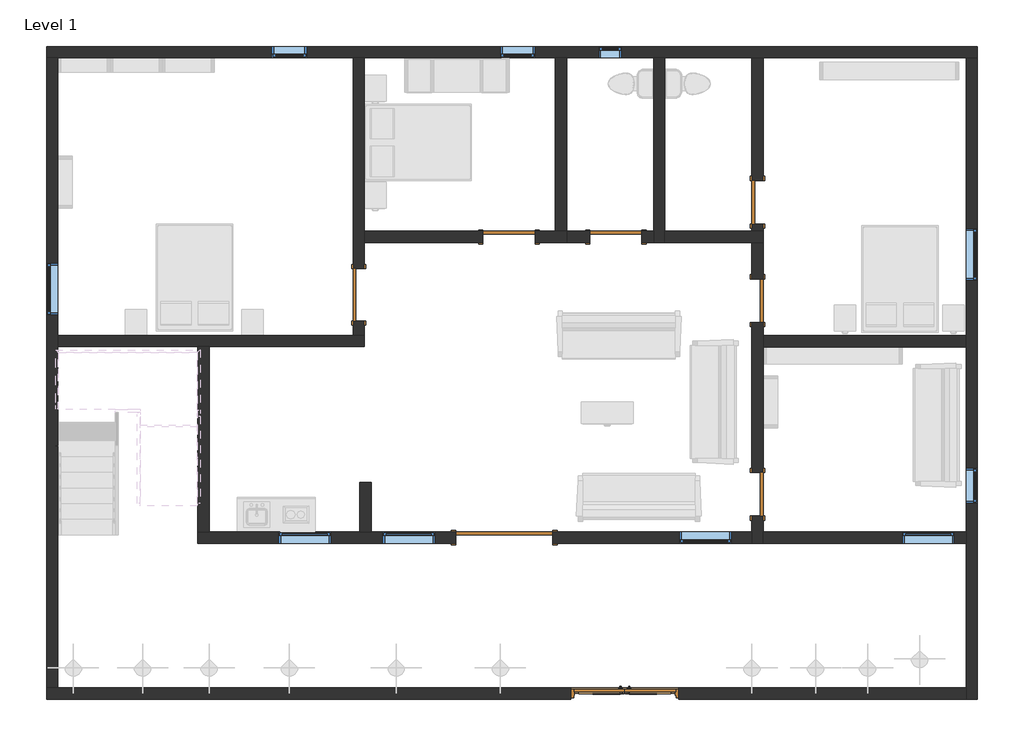
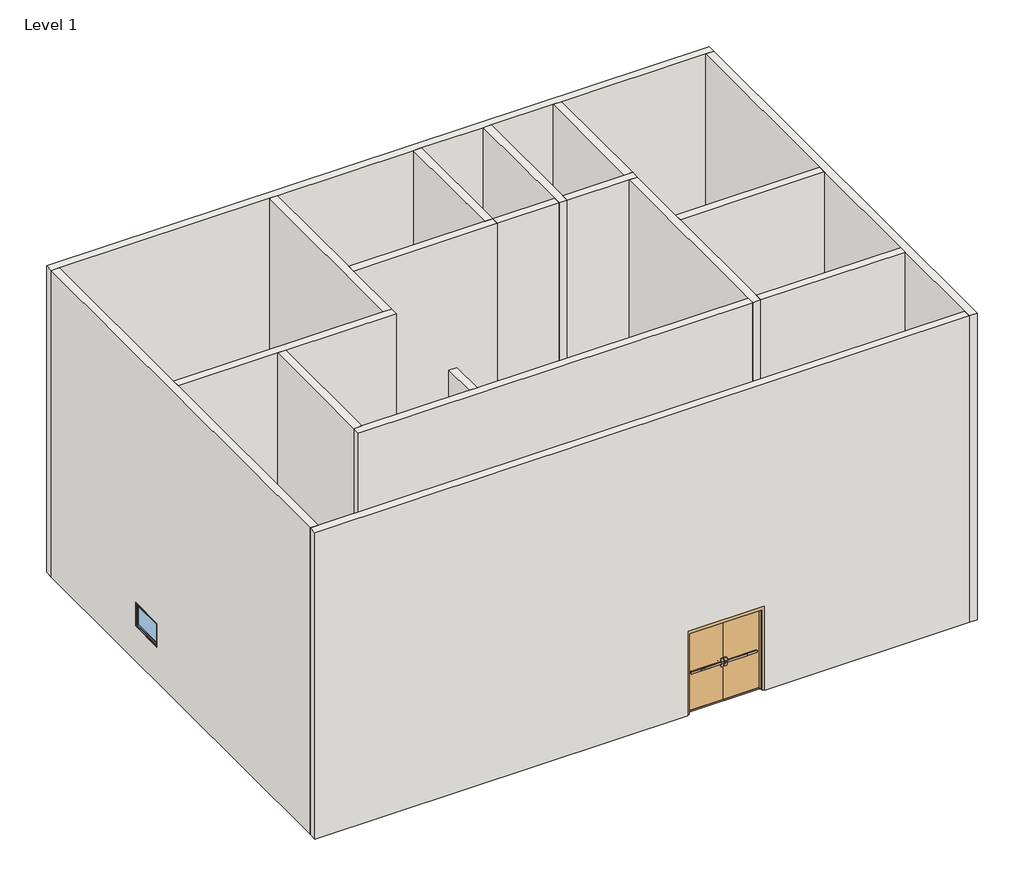
# One storey, part 1 of 4: 18 walls, 10 windows, 8 doors.
"""IFC4 building model written with IfcOpenShell, lengths in millimetres."""

from ifc_helpers import new_model, si_unit, frame, origin, origin_with_axes, place, context, project, spatial, polyline, outline, extrude, faceted_brep, transform, mapped, element, save
from components import m_door_double_flush_panel_double_acting_1700_x_2000mm_0a6d9c7f, m_door_exterior_double_m_door_exterior_double_5cdccef0, m_single_flush_0762_x_2032mm_7341a4fb, m_single_flush_0762_x_2032mm_0c256fab, m_single_flush_0915_x_2134mm_727434cd, m_single_flush_0915_x_2134mm_6a9e8738, m_fixed_0406_x_0610mm_8205b201, m_fixed_0610_x_0610mm_cacddef9, m_fixed_0610_x_1220mm_4e981104, m_fixed_0915_x_0610mm_70a843a6, m_fixed_0915_x_1830mm_5d6e8bc1

model = new_model("IFC4")

# Units and contexts
model_context = context("Model", 3, world=origin())
ifc_project = project(units=[si_unit("LENGTHUNIT", "METRE", prefix="MILLI")], contexts=[model_context])

# Site, building, storey
site = spatial("IfcSite", under=ifc_project)
building = spatial("IfcBuilding", under=site)
storey = spatial("IfcBuildingStorey", under=building, Name="Level 1", Elevation=0.0)

# Doors
placement = place(None, origin())
m_door_double_flush_panel_double_acting_1700_x_2000mm_shape = m_door_double_flush_panel_double_acting_1700_x_2000mm_0a6d9c7f(model_context)
element("IfcDoor", 1, ObjectType="M_Door-Double-Flush_Panel-Double-Acting : 1700 x 2000mm", at=placement, inside=storey, context=model_context, shape_type="MappedRepresentation", body=[
    mapped(m_door_double_flush_panel_double_acting_1700_x_2000mm_shape, transform((-4189.5676775, 775.0280728, 0.0), x_axis=(1.0, 0.0, 0.0), y_axis=(0.0, 1.0, 0.0), z_axis=(0.0, 0.0, 1.0))),
])
m_door_exterior_double_m_door_exterior_double_shape = m_door_exterior_double_m_door_exterior_double_5cdccef0(model_context)
element("IfcDoor", 2, ObjectType="M_Door-Exterior-Double : M_Door-Exterior-Double", at=placement, inside=storey, context=model_context, shape_type="MappedRepresentation", body=[
    mapped(m_door_exterior_double_m_door_exterior_double_shape, transform((-2073.3676775, -1974.5219272, 0.0), x_axis=(1.0, 0.0, 0.0), y_axis=(0.0, 1.0, 0.0), z_axis=(0.0, 0.0, 1.0))),
])
m_single_flush_0762_x_2032mm_shape = m_single_flush_0762_x_2032mm_7341a4fb(model_context)
element("IfcDoor", 3, ObjectType="M_Single-Flush : 0762 x 2032mm", at=placement, inside=storey, context=model_context, shape_type="MappedRepresentation", body=[
    mapped(m_single_flush_0762_x_2032mm_shape, transform((260.2323225, 6671.0280728, 0.0), x_axis=(0.0, -1.0, 0.0), y_axis=(1.0, 0.0, 0.0), z_axis=(0.0, 0.0, 1.0))),
])
m_single_flush_0762_x_2032mm_2_shape = m_single_flush_0762_x_2032mm_0c256fab(model_context)
element("IfcDoor", 4, ObjectType="M_Single-Flush : 0762 x 2032mm", at=placement, inside=storey, context=model_context, shape_type="MappedRepresentation", body=[
    mapped(m_single_flush_0762_x_2032mm_2_shape, transform((258.6323225, 4940.6280728, 0.0), x_axis=(0.0, -1.0, 0.0), y_axis=(1.0, 0.0, 0.0), z_axis=(0.0, 0.0, 1.0))),
])
element("IfcDoor", 5, ObjectType="M_Single-Flush : 0762 x 2032mm", at=placement, inside=storey, context=model_context, shape_type="MappedRepresentation", body=[
    mapped(m_single_flush_0762_x_2032mm_2_shape, transform((258.6323225, 1537.0280728, 0.0), x_axis=(0.0, -1.0, 0.0), y_axis=(1.0, 0.0, 0.0), z_axis=(0.0, 0.0, 1.0))),
])
m_single_flush_0915_x_2134mm_shape = m_single_flush_0915_x_2134mm_727434cd(model_context)
element("IfcDoor", 6, ObjectType="M_Single-Flush : 0915 x 2134mm", at=placement, inside=storey, context=model_context, shape_type="MappedRepresentation", body=[
    mapped(m_single_flush_0915_x_2134mm_shape, transform((-6746.9676775, 5043.8280728, 0.0), x_axis=(0.0, -1.0, 0.0), y_axis=(1.0, 0.0, 0.0), z_axis=(0.0, 0.0, 1.0))),
])
m_single_flush_0915_x_2134mm_2_shape = m_single_flush_0915_x_2134mm_6a9e8738(model_context)
element("IfcDoor", 7, ObjectType="M_Single-Flush : 0915 x 2134mm", at=placement, inside=storey, context=model_context, shape_type="MappedRepresentation", body=[
    mapped(m_single_flush_0915_x_2134mm_2_shape, transform((-4106.9676775, 6060.6280728, 0.0), x_axis=(1.0, 0.0, 0.0), y_axis=(0.0, 1.0, 0.0), z_axis=(0.0, 0.0, 1.0))),
])
element("IfcDoor", 8, ObjectType="M_Single-Flush : 0915 x 2134mm", at=placement, inside=storey, context=model_context, shape_type="MappedRepresentation", body=[
    mapped(m_single_flush_0915_x_2134mm_2_shape, transform((-2228.9676775, 6061.4280728, 0.0), x_axis=(1.0, 0.0, 0.0), y_axis=(0.0, 1.0, 0.0), z_axis=(0.0, 0.0, 1.0))),
])

# Walls
element("IfcWall", 9, ObjectType="Generic - 200mm", at=placement, inside=storey, context=model_context, shape_type="Brep", body=[
    faceted_brep([(-12231.7676775, 9209.4280728, 0.0), (-12031.7676775, 9209.4280728, 0.0), (-6846.9676775, 9209.4280728, 0.0), (-6646.9676775, 9209.4280728, 0.0), (-3292.5676775, 9209.4280728, 0.0), (-3092.5676775, 9209.4280728, 0.0), (-1566.9676775, 9209.4280728, 0.0), (-1366.9676775, 9209.4280728, 0.0), (160.2323225, 9209.4280728, 0.0), (360.2323225, 9209.4280728, 0.0), (3922.6323225, 9209.4280728, 0.0), (4122.6323225, 9209.4280728, 0.0), (4122.6323225, 9209.4280728, 8000.0), (3922.6323225, 9209.4280728, 8000.0), (360.2323225, 9209.4280728, 8000.0), (160.2323225, 9209.4280728, 8000.0), (-1366.9676775, 9209.4280728, 8000.0), (-1566.9676775, 9209.4280728, 8000.0), (-3092.5676775, 9209.4280728, 8000.0), (-3292.5676775, 9209.4280728, 8000.0), (-6646.9676775, 9209.4280728, 8000.0), (-6846.9676775, 9209.4280728, 8000.0), (-12031.7676775, 9209.4280728, 8000.0), (-12231.7676775, 9209.4280728, 8000.0), (-7661.1676775, 9209.4280728, 915.0), (-8271.1676775, 9209.4280728, 915.0), (-8271.1676775, 9209.4280728, 1525.0), (-7661.1676775, 9209.4280728, 1525.0), (-3649.5676775, 9209.4280728, 915.0), (-4259.5676775, 9209.4280728, 915.0), (-4259.5676775, 9209.4280728, 1525.0), (-3649.5676775, 9209.4280728, 1525.0), (-2532.7676775, 9209.4280728, 915.0), (-2532.7676775, 9209.4280728, 1525.0), (-2126.7676775, 9209.4280728, 1525.0), (-2126.7676775, 9209.4280728, 915.0), (-12231.7676775, 9409.4280728, 0.0), (-12231.7676775, 9409.4280728, 8000.0), (4122.6323225, 9409.4280728, 8000.0), (4122.6323225, 9409.4280728, 0.0), (-7661.1676775, 9409.4280728, 915.0), (-7661.1676775, 9409.4280728, 1525.0), (-8271.1676775, 9409.4280728, 1525.0), (-8271.1676775, 9409.4280728, 915.0), (-3649.5676775, 9409.4280728, 915.0), (-3649.5676775, 9409.4280728, 1525.0), (-4259.5676775, 9409.4280728, 1525.0), (-4259.5676775, 9409.4280728, 915.0), (-2532.7676775, 9409.4280728, 915.0), (-2126.7676775, 9409.4280728, 915.0), (-2126.7676775, 9409.4280728, 1525.0), (-2532.7676775, 9409.4280728, 1525.0)], [[[0, 1, 2, 3, 4, 5, 6, 7, 8, 9, 10, 11, 12, 13, 14, 15, 16, 17, 18, 19, 20, 21, 22, 23], [24, 25, 26, 27], [28, 29, 30, 31], [32, 33, 34, 35]], [[36, 37, 38, 39], [40, 41, 42, 43], [44, 45, 46, 47], [48, 49, 50, 51]], [[11, 10, 9, 8, 7, 6, 5, 4, 3, 2, 1, 0, 36, 39]], [[23, 22, 21, 20, 19, 18, 17, 16, 15, 14, 13, 12, 38, 37]], [[12, 11, 39, 38]], [[0, 23, 37, 36]], [[41, 40, 24, 27]], [[42, 41, 27, 26]], [[43, 42, 26, 25]], [[40, 43, 25, 24]], [[45, 44, 28, 31]], [[46, 45, 31, 30]], [[47, 46, 30, 29]], [[44, 47, 29, 28]], [[33, 32, 48, 51]], [[34, 33, 51, 50]], [[35, 34, 50, 49]], [[32, 35, 49, 48]]]),
])
element("IfcWall", 10, ObjectType="Generic - 200mm", at=placement, inside=storey, context=model_context, shape_type="Brep", body=[
    faceted_brep([(3922.6323225, 9209.4280728, 0.0), (3922.6323225, 4329.4280728, 0.0), (3922.6323225, 4129.4280728, 0.0), (3922.6323225, 875.0280728, 0.0), (3922.6323225, 675.0280728, 0.0), (3922.6323225, -1868.1719272, 0.0), (3922.6323225, -2068.1719272, 0.0), (3922.6323225, -2068.1719272, 8000.0), (3922.6323225, -1868.1719272, 8000.0), (3922.6323225, 675.0280728, 8000.0), (3922.6323225, 875.0280728, 8000.0), (3922.6323225, 4129.4280728, 8000.0), (3922.6323225, 4329.4280728, 8000.0), (3922.6323225, 9209.4280728, 8000.0), (3922.6323225, 1994.4280728, 915.0), (3922.6323225, 1994.4280728, 2135.0), (3922.6323225, 1384.4280728, 2135.0), (3922.6323225, 1384.4280728, 915.0), (3922.6323225, 6210.9280728, 915.0), (3922.6323225, 6210.9280728, 1525.0), (3922.6323225, 5295.9280728, 1525.0), (3922.6323225, 5295.9280728, 915.0), (4122.6323225, 9209.4280728, 0.0), (4122.6323225, 9209.4280728, 8000.0), (4122.6323225, -2068.1719272, 8000.0), (4122.6323225, -2068.1719272, 0.0), (4122.6323225, 1994.4280728, 915.0), (4122.6323225, 1384.4280728, 915.0), (4122.6323225, 1384.4280728, 2135.0), (4122.6323225, 1994.4280728, 2135.0), (4122.6323225, 6210.9280728, 915.0), (4122.6323225, 5295.9280728, 915.0), (4122.6323225, 5295.9280728, 1525.0), (4122.6323225, 6210.9280728, 1525.0)], [[[0, 1, 2, 3, 4, 5, 6, 7, 8, 9, 10, 11, 12, 13], [14, 15, 16, 17], [18, 19, 20, 21]], [[22, 23, 24, 25], [26, 27, 28, 29], [30, 31, 32, 33]], [[6, 5, 4, 3, 2, 1, 0, 22, 25]], [[13, 12, 11, 10, 9, 8, 7, 24, 23]], [[0, 13, 23, 22]], [[7, 6, 25, 24]], [[15, 14, 26, 29]], [[16, 15, 29, 28]], [[17, 16, 28, 27]], [[14, 17, 27, 26]], [[19, 18, 30, 33]], [[20, 19, 33, 32]], [[21, 20, 32, 31]], [[18, 21, 31, 30]]]),
])
element("IfcWall", 11, ObjectType="Generic - 200mm", at=placement, inside=storey, context=model_context, shape_type="Brep", body=[
    faceted_brep([(-12231.7676775, -1868.1719272, 8000.0), (-12031.7676775, -1868.1719272, 8000.0), (3922.6323225, -1868.1719272, 8000.0), (3922.6323225, -1868.1719272, 0.0), (-1123.3676775, -1868.1719272, 0.0), (-1123.3676775, -1868.1719272, 2200.0), (-3023.3676775, -1868.1719272, 2200.0), (-3023.3676775, -1868.1719272, 0.0), (-12031.7676775, -1868.1719272, 0.0), (-12231.7676775, -1868.1719272, 0.0), (3922.6323225, -2068.1719272, 8000.0), (-12231.7676775, -2068.1719272, 8000.0), (-12231.7676775, -2068.1719272, 0.0), (-3023.3676775, -2068.1719272, 0.0), (-3023.3676775, -2068.1719272, 2200.0), (-1123.3676775, -2068.1719272, 2200.0), (-1123.3676775, -2068.1719272, 0.0), (3922.6323225, -2068.1719272, 0.0)], [[[0, 1, 2, 3, 4, 5, 6, 7, 8, 9]], [[10, 11, 12, 13, 14, 15, 16, 17]], [[3, 17, 16, 4]], [[12, 9, 8, 7, 13]], [[2, 1, 0, 11, 10]], [[3, 2, 10, 17]], [[0, 9, 12, 11]], [[15, 5, 4, 16]], [[5, 15, 14, 6]], [[6, 14, 13, 7]]]),
])
element("IfcWall", 12, ObjectType="Generic - 200mm", at=placement, inside=storey, context=model_context, shape_type="Brep", body=[
    faceted_brep([(-12031.7676775, -1868.1719272, 0.0), (-12031.7676775, 4131.0280728, 0.0), (-12031.7676775, 4331.0280728, 0.0), (-12031.7676775, 9209.4280728, 0.0), (-12031.7676775, 9209.4280728, 8000.0), (-12031.7676775, 4331.0280728, 8000.0), (-12031.7676775, 4131.0280728, 8000.0), (-12031.7676775, -1868.1719272, 8000.0), (-12031.7676775, 4687.9280728, 915.0), (-12031.7676775, 4687.9280728, 1525.0), (-12031.7676775, 5602.9280728, 1525.0), (-12031.7676775, 5602.9280728, 915.0), (-12231.7676775, -1868.1719272, 0.0), (-12231.7676775, -1868.1719272, 8000.0), (-12231.7676775, 9209.4280728, 8000.0), (-12231.7676775, 9209.4280728, 0.0), (-12231.7676775, 4687.9280728, 915.0), (-12231.7676775, 5602.9280728, 915.0), (-12231.7676775, 5602.9280728, 1525.0), (-12231.7676775, 4687.9280728, 1525.0)], [[[0, 1, 2, 3, 4, 5, 6, 7], [8, 9, 10, 11]], [[12, 13, 14, 15], [16, 17, 18, 19]], [[3, 2, 1, 0, 12, 15]], [[7, 6, 5, 4, 14, 13]], [[0, 7, 13, 12]], [[4, 3, 15, 14]], [[9, 8, 16, 19]], [[10, 9, 19, 18]], [[11, 10, 18, 17]], [[8, 11, 17, 16]]]),
])
element("IfcWall", 13, ObjectType="Generic - 200mm", at=placement, inside=storey, context=model_context, shape_type="Brep", body=[
    faceted_brep([(-12031.7676775, 4131.0280728, 0.0), (-9575.9676775, 4131.0280728, 0.0), (-9375.9676775, 4131.0280728, 0.0), (-6646.9676775, 4131.0280728, 0.0), (-6646.9676775, 4131.0280728, 8000.0), (-9375.9676775, 4131.0280728, 8000.0), (-9575.9676775, 4131.0280728, 8000.0), (-12031.7676775, 4131.0280728, 8000.0), (-12031.7676775, 4331.0280728, 0.0), (-12031.7676775, 4331.0280728, 8000.0), (-6846.9676775, 4331.0280728, 8000.0), (-6646.9676775, 4331.0280728, 8000.0), (-6646.9676775, 4331.0280728, 0.0), (-6846.9676775, 4331.0280728, 0.0)], [[[0, 1, 2, 3, 4, 5, 6, 7]], [[8, 9, 10, 11, 12, 13]], [[3, 2, 1, 0, 8, 13, 12]], [[7, 6, 5, 4, 11, 10, 9]], [[4, 3, 12, 11]], [[0, 7, 9, 8]]]),
])
element("IfcWall", 14, ObjectType="Generic - 200mm", at=placement, inside=storey, context=model_context, shape_type="Brep", body=[
    faceted_brep([(-6646.9676775, 4331.0280728, 0.0), (-6646.9676775, 4586.3280728, 0.0), (-6646.9676775, 4586.3280728, 2134.0), (-6646.9676775, 5501.3280728, 2134.0), (-6646.9676775, 5501.3280728, 0.0), (-6646.9676775, 5960.6280728, 0.0), (-6646.9676775, 6160.6280728, 0.0), (-6646.9676775, 9209.4280728, 0.0), (-6646.9676775, 9209.4280728, 8000.0), (-6646.9676775, 6160.6280728, 8000.0), (-6646.9676775, 5960.6280728, 8000.0), (-6646.9676775, 4331.0280728, 8000.0), (-6846.9676775, 4586.3280728, 2134.0), (-6846.9676775, 4586.3280728, 0.0), (-6846.9676775, 4331.0280728, 0.0), (-6846.9676775, 4331.0280728, 8000.0), (-6846.9676775, 9209.4280728, 8000.0), (-6846.9676775, 9209.4280728, 0.0), (-6846.9676775, 5501.3280728, 0.0), (-6846.9676775, 5501.3280728, 2134.0)], [[[0, 1, 2, 3, 4, 5, 6, 7, 8, 9, 10, 11]], [[12, 13, 14, 15, 16, 17, 18, 19]], [[18, 17, 7, 6, 5, 4]], [[14, 13, 1, 0]], [[11, 10, 9, 8, 16, 15]], [[0, 11, 15, 14]], [[8, 7, 17, 16]], [[2, 1, 13, 12]], [[3, 2, 12, 19]], [[4, 3, 19, 18]]]),
])
element("IfcWall", 15, ObjectType="Generic - 200mm", at=placement, inside=storey, context=model_context, shape_type="Brep", body=[
    faceted_brep([(-3649.4676775, 5960.6280728, 2134.0), (-3649.4676775, 5960.6280728, 0.0), (-3092.5676775, 5960.6280728, 0.0), (-3092.5676775, 5960.6280728, 8000.0), (-6646.9676775, 5960.6280728, 8000.0), (-6646.9676775, 5960.6280728, 0.0), (-4564.4676775, 5960.6280728, 0.0), (-4564.4676775, 5960.6280728, 2134.0), (-3092.5676775, 6160.6280728, 0.0), (-3292.5676775, 6160.6280728, 0.0), (-3649.4676775, 6160.6280728, 0.0), (-3649.4676775, 6160.6280728, 2134.0), (-4564.4676775, 6160.6280728, 2134.0), (-4564.4676775, 6160.6280728, 0.0), (-6646.9676775, 6160.6280728, 0.0), (-6646.9676775, 6160.6280728, 8000.0), (-3292.5676775, 6160.6280728, 8000.0), (-3092.5676775, 6160.6280728, 8000.0), (-3092.5676775, 5961.4280728, 0.0), (-3092.5676775, 5961.4280728, 8000.0)], [[[0, 1, 2, 3, 4, 5, 6, 7]], [[8, 9, 10, 11, 12, 13, 14, 15, 16, 17]], [[6, 5, 14, 13]], [[2, 1, 10, 9, 8, 18]], [[4, 3, 19, 17, 16, 15]], [[5, 4, 15, 14]], [[3, 2, 18, 8, 17, 19]], [[11, 10, 1, 0]], [[12, 11, 0, 7]], [[13, 12, 7, 6]]]),
])
element("IfcWall", 16, ObjectType="Generic - 200mm", at=placement, inside=storey, context=model_context, shape_type="Brep", body=[
    faceted_brep([(-3092.5676775, 6160.6280728, 0.0), (-3092.5676775, 6161.4280728, 0.0), (-3092.5676775, 9209.4280728, 0.0), (-3092.5676775, 9209.4280728, 8000.0), (-3092.5676775, 6161.4280728, 8000.0), (-3092.5676775, 6160.6280728, 8000.0), (-3292.5676775, 6160.6280728, 0.0), (-3292.5676775, 6160.6280728, 8000.0), (-3292.5676775, 9209.4280728, 8000.0), (-3292.5676775, 9209.4280728, 0.0)], [[[0, 1, 2, 3, 4, 5]], [[6, 7, 8, 9]], [[2, 1, 0, 6, 9]], [[5, 4, 3, 8, 7]], [[0, 5, 7, 6]], [[3, 2, 9, 8]]]),
])
element("IfcWall", 17, ObjectType="Generic - 200mm", at=placement, inside=storey, context=model_context, shape_type="Brep", body=[
    faceted_brep([(-1566.9676775, 9209.4280728, 0.0), (-1566.9676775, 6161.4280728, 0.0), (-1566.9676775, 5961.4280728, 0.0), (-1566.9676775, 5961.4280728, 8000.0), (-1566.9676775, 6161.4280728, 8000.0), (-1566.9676775, 9209.4280728, 8000.0), (-1366.9676775, 9209.4280728, 0.0), (-1366.9676775, 9209.4280728, 8000.0), (-1366.9676775, 6161.4280728, 8000.0), (-1366.9676775, 5961.4280728, 8000.0), (-1366.9676775, 5961.4280728, 0.0), (-1366.9676775, 6161.4280728, 0.0)], [[[0, 1, 2, 3, 4, 5]], [[6, 7, 8, 9, 10, 11]], [[2, 1, 0, 6, 11, 10]], [[5, 4, 3, 9, 8, 7]], [[0, 5, 7, 6]], [[3, 2, 10, 9]]]),
])
element("IfcWall", 18, ObjectType="Generic - 200mm", at=placement, inside=storey, context=model_context, shape_type="Brep", body=[
    faceted_brep([(-1566.9676775, 6161.4280728, 0.0), (-1771.4676775, 6161.4280728, 0.0), (-1771.4676775, 6161.4280728, 2134.0), (-2686.4676775, 6161.4280728, 2134.0), (-2686.4676775, 6161.4280728, 0.0), (-3092.5676775, 6161.4280728, 0.0), (-3092.5676775, 6161.4280728, 8000.0), (-1566.9676775, 6161.4280728, 8000.0), (-1771.4676775, 5961.4280728, 2134.0), (-1771.4676775, 5961.4280728, 0.0), (-1566.9676775, 5961.4280728, 0.0), (-1566.9676775, 5961.4280728, 8000.0), (-3092.5676775, 5961.4280728, 8000.0), (-3092.5676775, 5961.4280728, 0.0), (-2686.4676775, 5961.4280728, 0.0), (-2686.4676775, 5961.4280728, 2134.0), (-3092.5676775, 6160.6280728, 0.0), (-3092.5676775, 6160.6280728, 8000.0)], [[[0, 1, 2, 3, 4, 5, 6, 7]], [[8, 9, 10, 11, 12, 13, 14, 15]], [[14, 13, 16, 5, 4]], [[10, 9, 1, 0]], [[7, 6, 17, 12, 11]], [[0, 7, 11, 10]], [[6, 5, 16, 13, 12, 17]], [[2, 1, 9, 8]], [[3, 2, 8, 15]], [[4, 3, 15, 14]]]),
])
element("IfcWall", 19, ObjectType="Generic - 200mm", at=placement, inside=storey, context=model_context, shape_type="Brep", body=[
    faceted_brep([(-1366.9676775, 5961.4280728, 0.0), (158.6323225, 5961.4280728, 0.0), (358.6323225, 5961.4280728, 0.0), (360.2323225, 5961.4280728, 0.0), (360.2323225, 5961.4280728, 8000.0), (358.6323225, 5961.4280728, 8000.0), (158.6323225, 5961.4280728, 8000.0), (-1366.9676775, 5961.4280728, 8000.0), (-1366.9676775, 6161.4280728, 0.0), (-1366.9676775, 6161.4280728, 8000.0), (160.2323225, 6161.4280728, 8000.0), (360.2323225, 6161.4280728, 8000.0), (360.2323225, 6161.4280728, 0.0), (160.2323225, 6161.4280728, 0.0)], [[[0, 1, 2, 3, 4, 5, 6, 7]], [[8, 9, 10, 11, 12, 13]], [[3, 2, 1, 0, 8, 13, 12]], [[7, 6, 5, 4, 11, 10, 9]], [[0, 7, 9, 8]], [[4, 3, 12, 11]]]),
])
element("IfcWall", 20, ObjectType="Generic - 200mm", at=placement, inside=storey, context=model_context, shape_type="SweptSolid", body=[
    extrude(outline(polyline([(6290.0280728, 2032.0), (6290.0280728, 0.0), (6161.4280728, 0.0), (6161.4280728, 8000.0), (9209.4280728, 8000.0), (9209.4280728, 0.0), (7052.0280728, 0.0), (7052.0280728, 2032.0), (6290.0280728, 2032.0)])), frame((160.2323225, 0.0, 0.0), z_axis=(1.0, 0.0, 0.0), x_axis=(0.0, 1.0, 0.0)), (0.0, 0.0, 1.0), 200.0),
])
element("IfcWall", 21, ObjectType="Generic - 200mm", at=placement, inside=storey, context=model_context, shape_type="SweptSolid", body=[
    extrude(outline(polyline([(3922.6323225, 4129.4280728), (358.6323225, 4129.4280728), (358.6323225, 4329.4280728), (3922.6323225, 4329.4280728), (3922.6323225, 4129.4280728)])), origin_with_axes(), (0.0, 0.0, 1.0), 8000.0),
])
element("IfcWall", 22, ObjectType="Generic - 200mm", at=placement, inside=storey, context=model_context, shape_type="Brep", body=[
    faceted_brep([(158.6323225, 1156.0280728, 2032.0), (158.6323225, 1156.0280728, 0.0), (158.6323225, 875.0280728, 0.0), (158.6323225, 675.0280728, 0.0), (158.6323225, 675.0280728, 8000.0), (158.6323225, 875.0280728, 8000.0), (158.6323225, 5961.4280728, 8000.0), (158.6323225, 5961.4280728, 0.0), (158.6323225, 5321.6280728, 0.0), (158.6323225, 5321.6280728, 2032.0), (158.6323225, 4559.6280728, 2032.0), (158.6323225, 4559.6280728, 0.0), (158.6323225, 1918.0280728, 0.0), (158.6323225, 1918.0280728, 2032.0), (358.6323225, 675.0280728, 0.0), (358.6323225, 875.0280728, 0.0), (358.6323225, 1156.0280728, 0.0), (358.6323225, 1156.0280728, 2032.0), (358.6323225, 1918.0280728, 2032.0), (358.6323225, 1918.0280728, 0.0), (358.6323225, 4129.4280728, 0.0), (358.6323225, 4329.4280728, 0.0), (358.6323225, 4559.6280728, 0.0), (358.6323225, 4559.6280728, 2032.0), (358.6323225, 5321.6280728, 2032.0), (358.6323225, 5321.6280728, 0.0), (358.6323225, 5961.4280728, 0.0), (358.6323225, 5961.4280728, 8000.0), (358.6323225, 4329.4280728, 8000.0), (358.6323225, 4129.4280728, 8000.0), (358.6323225, 875.0280728, 8000.0), (358.6323225, 675.0280728, 8000.0)], [[[0, 1, 2, 3, 4, 5, 6, 7, 8, 9, 10, 11, 12, 13]], [[14, 15, 16, 17, 18, 19, 20, 21, 22, 23, 24, 25, 26, 27, 28, 29, 30, 31]], [[8, 7, 26, 25]], [[12, 11, 22, 21, 20, 19]], [[3, 2, 1, 16, 15, 14]], [[6, 5, 4, 31, 30, 29, 28, 27]], [[7, 6, 27, 26]], [[23, 22, 11, 10]], [[24, 23, 10, 9]], [[25, 24, 9, 8]], [[4, 3, 14, 31]], [[17, 16, 1, 0]], [[18, 17, 0, 13]], [[19, 18, 13, 12]]]),
])
element("IfcWall", 23, ObjectType="Generic - 200mm", at=placement, inside=storey, context=model_context, shape_type="SweptSolid", body=[
    extrude(outline(polyline([(0.0, 358.6323225), (0.0, 3922.6323225), (8000.0, 3922.6323225), (8000.0, 358.6323225), (0.0, 358.6323225)]), holes=[polyline([(915.0, 2803.1323225), (1525.0, 2803.1323225), (1525.0, 3718.1323225), (915.0, 3718.1323225), (915.0, 2803.1323225)])]), frame((0.0, 675.0280728, 0.0), z_axis=(0.0, 1.0, 0.0), x_axis=(0.0, 0.0, 1.0)), (0.0, 0.0, 1.0), 200.0),
])
element("IfcWall", 24, ObjectType="Generic - 200mm", at=placement, inside=storey, context=model_context, shape_type="Brep", body=[
    faceted_brep([(-9575.9676775, 875.0280728, 8000.0), (-9375.9676775, 875.0280728, 8000.0), (-6727.9676775, 875.0280728, 8000.0), (-6527.9676775, 875.0280728, 8000.0), (158.6323225, 875.0280728, 8000.0), (158.6323225, 875.0280728, 0.0), (-3339.5676775, 875.0280728, 0.0), (-3339.5676775, 875.0280728, 2000.0), (-5039.5676775, 875.0280728, 2000.0), (-5039.5676775, 875.0280728, 0.0), (-6527.9676775, 875.0280728, 0.0), (-6727.9676775, 875.0280728, 0.0), (-9375.9676775, 875.0280728, 0.0), (-9575.9676775, 875.0280728, 0.0), (-8152.2676775, 875.0280728, 915.0), (-7237.2676775, 875.0280728, 915.0), (-7237.2676775, 875.0280728, 1525.0), (-8152.2676775, 875.0280728, 1525.0), (-6323.4676775, 875.0280728, 305.0), (-5408.4676775, 875.0280728, 305.0), (-5408.4676775, 875.0280728, 2135.0), (-6323.4676775, 875.0280728, 2135.0), (-198.2676775, 875.0280728, 305.0), (-198.2676775, 875.0280728, 2135.0), (-1113.2676775, 875.0280728, 2135.0), (-1113.2676775, 875.0280728, 305.0), (158.6323225, 675.0280728, 8000.0), (-9575.9676775, 675.0280728, 8000.0), (-9575.9676775, 675.0280728, 0.0), (-5039.5676775, 675.0280728, 0.0), (-5039.5676775, 675.0280728, 2000.0), (-3339.5676775, 675.0280728, 2000.0), (-3339.5676775, 675.0280728, 0.0), (158.6323225, 675.0280728, 0.0), (-8152.2676775, 675.0280728, 915.0), (-8152.2676775, 675.0280728, 1525.0), (-7237.2676775, 675.0280728, 1525.0), (-7237.2676775, 675.0280728, 915.0), (-6323.4676775, 675.0280728, 305.0), (-6323.4676775, 675.0280728, 2135.0), (-5408.4676775, 675.0280728, 2135.0), (-5408.4676775, 675.0280728, 305.0), (-198.2676775, 675.0280728, 305.0), (-1113.2676775, 675.0280728, 305.0), (-1113.2676775, 675.0280728, 2135.0), (-198.2676775, 675.0280728, 2135.0)], [[[0, 1, 2, 3, 4, 5, 6, 7, 8, 9, 10, 11, 12, 13], [14, 15, 16, 17], [18, 19, 20, 21], [22, 23, 24, 25]], [[26, 27, 28, 29, 30, 31, 32, 33], [34, 35, 36, 37], [38, 39, 40, 41], [42, 43, 44, 45]], [[5, 33, 32, 6]], [[28, 13, 12, 11, 10, 9, 29]], [[4, 3, 2, 1, 0, 27, 26]], [[5, 4, 26, 33]], [[0, 13, 28, 27]], [[35, 34, 14, 17]], [[36, 35, 17, 16]], [[37, 36, 16, 15]], [[34, 37, 15, 14]], [[39, 38, 18, 21]], [[40, 39, 21, 20]], [[41, 40, 20, 19]], [[38, 41, 19, 18]], [[23, 22, 42, 45]], [[24, 23, 45, 44]], [[25, 24, 44, 43]], [[22, 25, 43, 42]], [[31, 7, 6, 32]], [[7, 31, 30, 8]], [[8, 30, 29, 9]]]),
])
element("IfcWall", 25, ObjectType="Generic - 200mm", at=placement, inside=storey, context=model_context, shape_type="SweptSolid", body=[
    extrude(outline(polyline([(-6527.9676775, 1741.8280728), (-6527.9676775, 875.0280728), (-6727.9676775, 875.0280728), (-6727.9676775, 1741.8280728), (-6527.9676775, 1741.8280728)])), origin_with_axes(), (0.0, 0.0, 1.0), 8000.0),
])
element("IfcWall", 26, ObjectType="Generic - 200mm", at=placement, inside=storey, context=model_context, shape_type="SweptSolid", body=[
    extrude(outline(polyline([(-9375.9676775, 4131.0280728), (-9375.9676775, 875.0280728), (-9575.9676775, 875.0280728), (-9575.9676775, 4131.0280728), (-9375.9676775, 4131.0280728)])), origin_with_axes(), (0.0, 0.0, 1.0), 8000.0),
])

# Windows
m_fixed_0406_x_0610mm_shape = m_fixed_0406_x_0610mm_8205b201(model_context)
element("IfcWindow", 27, ObjectType="M_Fixed : 0406 x 0610mm", at=placement, inside=storey, context=model_context, shape_type="MappedRepresentation", body=[
    mapped(m_fixed_0406_x_0610mm_shape, transform((-2329.7676775, 9296.4280728, 0.0), x_axis=(1.0, 0.0, 0.0), y_axis=(0.0, 1.0, 0.0), z_axis=(0.0, 0.0, 1.0))),
])
m_fixed_0610_x_0610mm_shape = m_fixed_0610_x_0610mm_cacddef9(model_context)
element("IfcWindow", 28, ObjectType="M_Fixed : 0610 x 0610mm", at=placement, inside=storey, context=model_context, shape_type="MappedRepresentation", body=[
    mapped(m_fixed_0610_x_0610mm_shape, transform((-7966.1676775, 9322.4280728, 0.0), x_axis=(-1.0, 0.0, 0.0), y_axis=(0.0, -1.0, 0.0), z_axis=(0.0, 0.0, 1.0))),
])
element("IfcWindow", 29, ObjectType="M_Fixed : 0610 x 0610mm", at=placement, inside=storey, context=model_context, shape_type="MappedRepresentation", body=[
    mapped(m_fixed_0610_x_0610mm_shape, transform((-3954.5676775, 9322.4280728, 0.0), x_axis=(-1.0, 0.0, 0.0), y_axis=(0.0, -1.0, 0.0), z_axis=(0.0, 0.0, 1.0))),
])
m_fixed_0610_x_1220mm_shape = m_fixed_0610_x_1220mm_4e981104(model_context)
element("IfcWindow", 30, ObjectType="M_Fixed : 0610 x 1220mm", at=placement, inside=storey, context=model_context, shape_type="MappedRepresentation", body=[
    mapped(m_fixed_0610_x_1220mm_shape, transform((4009.6323225, 1689.4280728, 0.0), x_axis=(0.0, -1.0, 0.0), y_axis=(1.0, 0.0, 0.0), z_axis=(0.0, 0.0, 1.0))),
])
m_fixed_0915_x_0610mm_shape = m_fixed_0915_x_0610mm_70a843a6(model_context)
element("IfcWindow", 31, ObjectType="M_Fixed : 0915 x 0610mm", at=placement, inside=storey, context=model_context, shape_type="MappedRepresentation", body=[
    mapped(m_fixed_0915_x_0610mm_shape, transform((4009.6323225, 5753.4280728, 0.0), x_axis=(0.0, -1.0, 0.0), y_axis=(1.0, 0.0, 0.0), z_axis=(0.0, 0.0, 1.0))),
])
element("IfcWindow", 32, ObjectType="M_Fixed : 0915 x 0610mm", at=placement, inside=storey, context=model_context, shape_type="MappedRepresentation", body=[
    mapped(m_fixed_0915_x_0610mm_shape, transform((3260.6323225, 762.0280728, 0.0), x_axis=(1.0, 0.0, 0.0), y_axis=(0.0, 1.0, 0.0), z_axis=(0.0, 0.0, 1.0))),
])
element("IfcWindow", 33, ObjectType="M_Fixed : 0915 x 0610mm", at=placement, inside=storey, context=model_context, shape_type="MappedRepresentation", body=[
    mapped(m_fixed_0915_x_0610mm_shape, transform((-7694.7676775, 762.0280728, 0.0), x_axis=(1.0, 0.0, 0.0), y_axis=(0.0, 1.0, 0.0), z_axis=(0.0, 0.0, 1.0))),
])
element("IfcWindow", 34, ObjectType="M_Fixed : 0915 x 0610mm", at=placement, inside=storey, context=model_context, shape_type="MappedRepresentation", body=[
    mapped(m_fixed_0915_x_0610mm_shape, transform((-12118.7676775, 5145.4280728, 0.0), x_axis=(0.0, 1.0, 0.0), y_axis=(-1.0, 0.0, 0.0), z_axis=(0.0, 0.0, 1.0))),
])
m_fixed_0915_x_1830mm_shape = m_fixed_0915_x_1830mm_5d6e8bc1(model_context)
element("IfcWindow", 35, ObjectType="M_Fixed : 0915 x 1830mm", at=placement, inside=storey, context=model_context, shape_type="MappedRepresentation", body=[
    mapped(m_fixed_0915_x_1830mm_shape, transform((-5865.9676775, 762.0280728, 0.0), x_axis=(1.0, 0.0, 0.0), y_axis=(0.0, 1.0, 0.0), z_axis=(0.0, 0.0, 1.0))),
])
element("IfcWindow", 36, ObjectType="M_Fixed : 0915 x 1830mm", at=placement, inside=storey, context=model_context, shape_type="MappedRepresentation", body=[
    mapped(m_fixed_0915_x_1830mm_shape, transform((-655.7676775, 788.0280728, 0.0), x_axis=(-1.0, 0.0, 0.0), y_axis=(0.0, -1.0, 0.0), z_axis=(0.0, 0.0, 1.0))),
])

save(model, "model.ifc")

# Revit data of these elements
# Type "M_Door-Double-Flush_Panel-Double-Acting : 1700 x 2000mm"
#   Type Mark = "22"
#   Construction Type Id = "DOOR"
#   Assembly Code = "C1020"
#   Analytic Construction = "Wooden"
#   W = 850 mm
#   Thickness = 50 mm
#   Thermal Resistance (R) = 0.455703 (m²·K)/W
#   Swing Angle [instance default] = 90.00°
#   Heat Transfer Coefficient (U) = 2.19465 W/(m²·K)
#   Height = 2000 mm
#   Trim Projection Ext. = 25 mm
#   Trim Projection Int. = 25 mm
#   Trim Width Ext. = 80 mm
#   Trim Width Int. = 80 mm
#   Width = 1700 mm
#   Define Thermal Properties by = 1
#   Panel Material = Wood - Birch - Solid Stained Light Low Gloss
#   Trim Material = Paint - Sienna
#   Visual Light Transmittance = 0
#   Solar Heat Gain Coefficient = 0
#   Function = (empty or 0)
#   Wall Closure = (empty or 0)
# Type "M_Door-Exterior-Double : M_Door-Exterior-Double"
#   Type Mark = "23"
#   Assembly Code = "B2030200"
#   Analytic Construction = "Metal"
#   Threshold Length [instance default] = 1900 mm
#   Threshold Offset [instance default] = 15 mm
#   Thickness = 45 mm
#   Thermal Resistance (R) = 0.270118 (m²·K)/W
#   Swing Angle [instance default] = 90.00°
#   Strike Height = 1000 mm
#   SinglePanelWidth = 900 mm
#   Rough Width [instance default] = 1900 mm
#   Rough Height [instance default] = 2200 mm
#   MFOpeningHeight [instance default] = 100 mm
#   MFOpeningWidth [instance default] = 100 mm
#   Inset Calculate [instance default] = 105 mm
#   Masonry Inset [instance default] = 25 mm
#   Height = 2100 mm
#   Width = 1800 mm
#   Heat Transfer Coefficient (U) = 3.70223 W/(m²·K)
#   Masonry Frame Depth = 150 mm
#   Threshold [instance default] = yes
#   Masonry Frame [instance default] = yes
#   Function = 1
#   Dry Wall Frame [instance default] = no
#   Threshold Material = Cherry
#   Panic Bar Material = Metal - Stainless Steel
#   Panel Material = Metal - Painted - Grey
#   Frame Material = Metal - Painted - Grey
#   Exterior Pull Material = Metal - Stainless Steel
#   Visual Light Transmittance = 0
#   Solar Heat Gain Coefficient = 0
#   Wall Closure = (empty or 0)
# Type "M_Single-Flush : 0762 x 2032mm"
#   Type Mark = "19"
#   Thickness = 51 mm
#   Height = 2032 mm
#   Trim Projection Ext = 25 mm
#   Trim Projection Int = 25 mm
#   Trim Width = 76 mm
#   Width = 762 mm
#   Door Material = Door - Panel
#   Frame Material = Door - Frame
#   Function = (empty or 0)
#   Wall Closure = (empty or 0)
# Type "M_Single-Flush : 0915 x 2134mm"
#   Type Mark = "15"
#   Thickness = 51 mm
#   Height = 2134 mm
#   Trim Projection Ext = 25 mm
#   Trim Projection Int = 25 mm
#   Trim Width = 76 mm
#   Width = 915 mm
#   Door Material = Door - Panel
#   Frame Material = Door - Frame
#   Function = (empty or 0)
#   Wall Closure = (empty or 0)
# Type "Generic - 200mm"
#   Layers, outside or top first: 200 mm no material (function 1)
# Type "M_Fixed : 0406 x 0610mm"
#   Type Mark = "10"
#   Height = 610 mm
#   Default Sill Height = 915 mm
#   Width = 406 mm
#   Window Inset = 19 mm
#   Frame Exterior Material = Sash
#   Frame Interior Material = Sash
#   Glass Pane Material = Glass
#   Sash = Sash
#   Wall Closure = (empty or 0)
# Type "M_Fixed : 0610 x 0610mm"
#   Type Mark = "12"
#   Height = 610 mm
#   Default Sill Height = 915 mm
#   Width = 610 mm
#   Window Inset = 19 mm
#   Frame Exterior Material = Sash
#   Frame Interior Material = Sash
#   Glass Pane Material = Glass
#   Sash = Sash
#   Wall Closure = (empty or 0)
# Type "M_Fixed : 0610 x 1220mm"
#   Type Mark = "13"
#   Height = 1220 mm
#   Default Sill Height = 915 mm
#   Width = 610 mm
#   Window Inset = 19 mm
#   Frame Exterior Material = Sash
#   Frame Interior Material = Sash
#   Glass Pane Material = Glass
#   Sash = Sash
#   Wall Closure = (empty or 0)
# Type "M_Fixed : 0915 x 0610mm"
#   Type Mark = "14"
#   Height = 610 mm
#   Default Sill Height = 915 mm
#   Width = 915 mm
#   Window Inset = 19 mm
#   Frame Exterior Material = Sash
#   Frame Interior Material = Sash
#   Glass Pane Material = Glass
#   Sash = Sash
#   Wall Closure = (empty or 0)
# Type "M_Fixed : 0915 x 1830mm"
#   Type Mark = "18"
#   Height = 1830 mm
#   Default Sill Height = 305 mm
#   Width = 915 mm
#   Window Inset = 19 mm
#   Frame Exterior Material = Sash
#   Frame Interior Material = Sash
#   Glass Pane Material = Glass
#   Sash = Sash
#   Wall Closure = (empty or 0)
# Element 1 (IfcDoor, "M_Door-Double-Flush_Panel-Double-Acting : 1700 x 2000mm")
#   Swing Angle = 90.00°
#   Phase Created = New Construction
#   Materials on its faces: "Paint - Sienna", "Wood - Birch - Solid Stained Light Low Gloss"
# Element 2 (IfcDoor, "M_Door-Exterior-Double : M_Door-Exterior-Double")
#   Threshold Offset = 15 mm
#   Threshold Length = 1900 mm
#   Swing Angle = 90.00°
#   Rough Width = 1900 mm
#   Rough Height = 2200 mm
#   Masonry Inset = 25 mm
#   MFOpeningWidth = 100 mm
#   MFOpeningHeight = 100 mm
#   Inset Calculate = 105 mm
#   Threshold = yes
#   Masonry Frame = yes
#   Dry Wall Frame = no
#   Phase Created = New Construction
#   Materials on its faces: "Metal - Stainless Steel", "Metal - Painted - Grey", "Cherry"
# Elements 3, 4, 5 (IfcDoor, "M_Single-Flush : 0762 x 2032mm")
#   Phase Created = New Construction
#   Materials on its faces: "Door - Frame", "Door - Panel"
# Elements 6, 7, 8 (IfcDoor, "M_Single-Flush : 0915 x 2134mm")
#   Phase Created = New Construction
#   Materials on its faces: "Door - Frame", "Door - Panel"
# Elements 9, 10, 11, 12, 13, 14, 15, 16, 17, 18, 19, 20, 21, 22, 23, 24, 25, 26 (IfcWall, "Generic - 200mm")
#   Top Offset = 0 mm
#   Base Offset = 0 mm
#   Unconnected Height = 8000 mm
#   wall height = 8000 mm
#   Phase Created = New Construction
#   Base Constraint = Level 1
#   Materials on its faces: "Default Wall"
# Element 27 (IfcWindow, "M_Fixed : 0406 x 0610mm")
#   Mark = "8"
#   Phase Created = New Construction
#   Materials on its faces: "Sash", "Glass"
# Element 28 (IfcWindow, "M_Fixed : 0610 x 0610mm")
#   Mark = "6"
#   Phase Created = New Construction
#   Materials on its faces: "Sash", "Glass"
# Element 29 (IfcWindow, "M_Fixed : 0610 x 0610mm")
#   Mark = "7"
#   Phase Created = New Construction
#   Materials on its faces: "Sash", "Glass"
# Element 30 (IfcWindow, "M_Fixed : 0610 x 1220mm")
#   Mark = "9"
#   Phase Created = New Construction
#   Materials on its faces: "Sash", "Glass"
# Element 31 (IfcWindow, "M_Fixed : 0915 x 0610mm")
#   Mark = "10"
#   Phase Created = New Construction
#   Materials on its faces: "Sash", "Glass"
# Element 32 (IfcWindow, "M_Fixed : 0915 x 0610mm")
#   Mark = "11"
#   Phase Created = New Construction
#   Materials on its faces: "Sash", "Glass"
# Element 33 (IfcWindow, "M_Fixed : 0915 x 0610mm")
#   Mark = "12"
#   Phase Created = New Construction
#   Materials on its faces: "Sash", "Glass"
# Element 34 (IfcWindow, "M_Fixed : 0915 x 0610mm")
#   Mark = "13"
#   Phase Created = New Construction
#   Materials on its faces: "Sash", "Glass"
# Element 35 (IfcWindow, "M_Fixed : 0915 x 1830mm")
#   Mark = "14"
#   Phase Created = New Construction
#   Materials on its faces: "Sash", "Glass"
# Element 36 (IfcWindow, "M_Fixed : 0915 x 1830mm")
#   Mark = "15"
#   Phase Created = New Construction
#   Materials on its faces: "Sash", "Glass"
# Materials
#   "Wood - Birch - Solid Stained Light Low Gloss": class "Wood", colour RGB 210 159 95, transparency 0, Cost = 0
#   "Paint - Sienna": colour RGB 118 70 51, transparency 0, Cost = 0
#   "Cherry": class "Wood", colour RGB 154 107 61, transparency 0, Description = "Prunus Serotina", Cost = 0
#   "Metal - Stainless Steel": class "Metal", colour RGB 247 247 247, transparency 0
#   "Metal - Painted - Grey": class "Paint", colour RGB 104 104 104, transparency 0, Cost = 0
#   "Door - Panel": class "Wood", colour RGB 114 82 51, transparency 0
#   "Door - Frame": colour RGB 153 76 43, transparency 0
#   "Sash": class "Wood", colour RGB 136 99 55, transparency 0
#   "Glass": class "Glass", colour RGB 218 227 224, transparency 0.85, Description = "Soda Lime Glass", Cost = 0
#   "Default Wall": colour RGB 80 80 80, transparency 0
